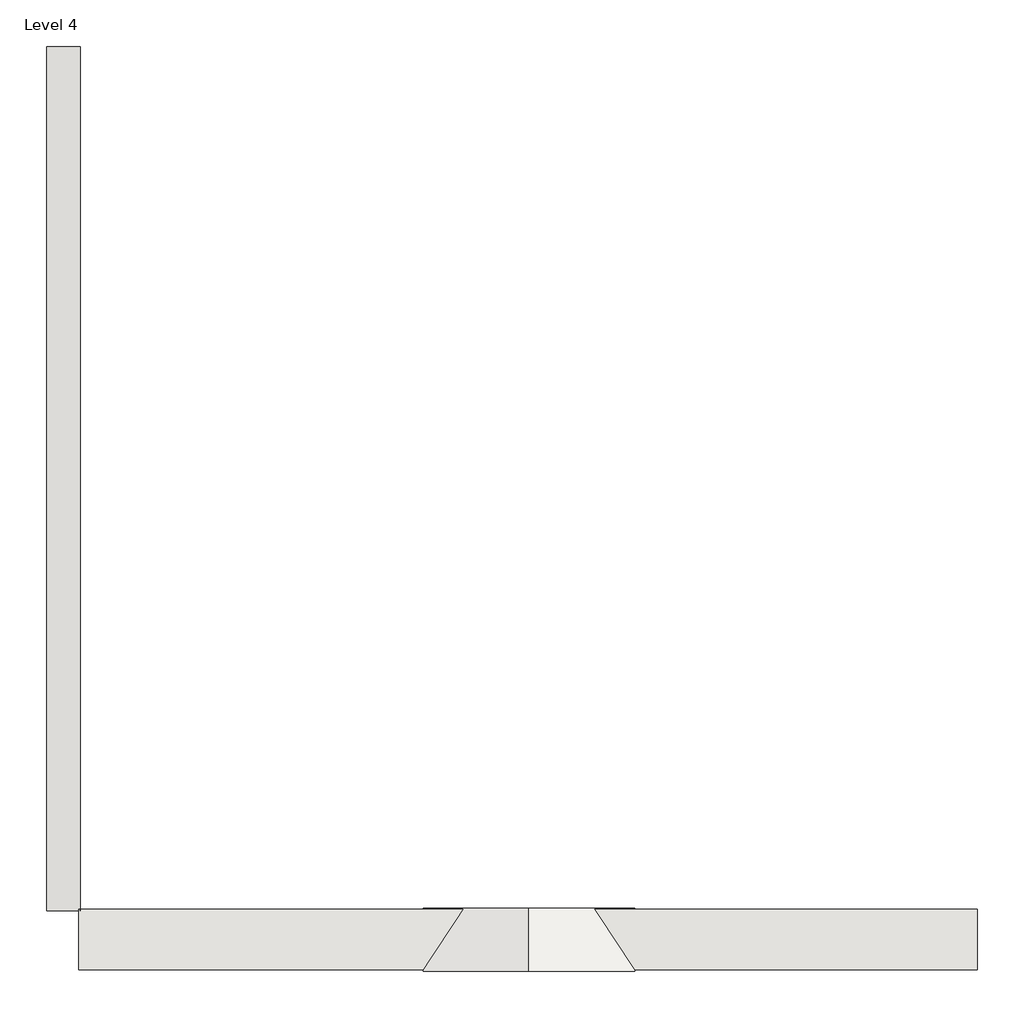
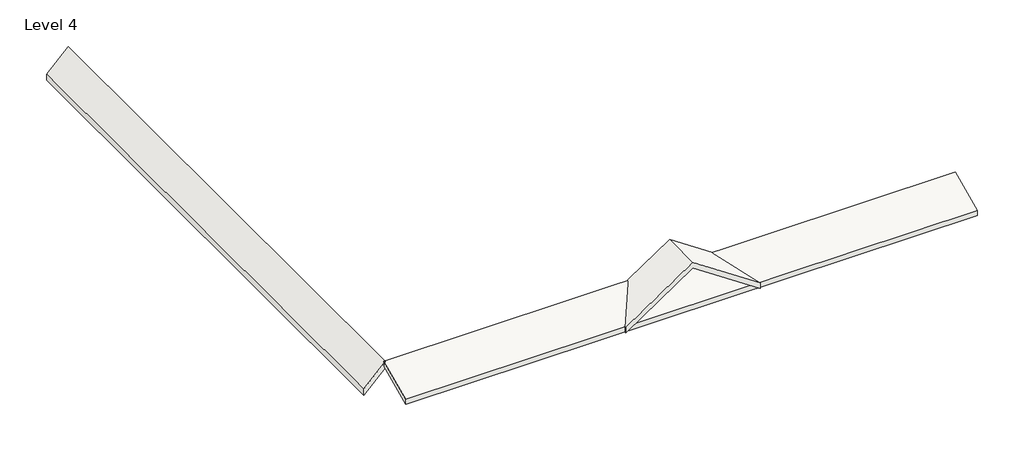
# One storey: 3 roofs.
"""IFC4 building model written with IfcOpenShell, lengths in millimetres."""

from ifc_helpers import new_model, si_unit, frame, origin, place, context, project, spatial, polyline, outline, extrude, element, save

model = new_model("IFC4")

# Units and contexts
model_context = context("Model", 3, world=origin())
ifc_project = project(units=[si_unit("LENGTHUNIT", "METRE", prefix="MILLI")], contexts=[model_context])

# Site, building, storey
site = spatial("IfcSite", under=ifc_project)
building = spatial("IfcBuilding", under=site)
storey = spatial("IfcBuildingStorey", under=building, Name="Level 4", Elevation=6858.0)

# Roofs
placement = place(None, origin())
element("IfcRoof", 1, ObjectType="6\" roof", at=placement, inside=storey, context=model_context, shape_type="SweptSolid", body=[
    extrude(outline(polyline([(-10080.7067839, 3252.1200204), (-8827.6878342, 3810.0), (-8827.6878342, 3643.1774312), (-10080.7067839, 3085.2974515), (-10080.7067839, 3252.1200204)])), frame((-9809.6634433, 0.0, 0.0), z_axis=(1.0, 0.0, 0.0), x_axis=(0.0, 1.0, 0.0)), (0.0, 0.0, 1.0), 18555.8213774),
])
element("IfcRoof", 2, ObjectType="6\" roof", at=placement, inside=storey, context=model_context, shape_type="SweptSolid", body=[
    extrude(outline(polyline([(3252.1200204, -2694.8868984), (3068.292405, -2694.8868984), (4540.5723846, -512.1420659), (3068.292405, 1670.6027667), (3252.1200204, 1670.6027667), (4724.4, -512.1420659), (3252.1200204, -2694.8868984)])), frame((0.0, -10112.12759, 0.0), z_axis=(0.0, 1.0, 0.0), x_axis=(0.0, 0.0, 1.0)), (0.0, 0.0, 1.0), 1298.9023851),
])
element("IfcRoof", 3, ObjectType="6\" roof", at=placement, inside=storey, context=model_context, shape_type="SweptSolid", body=[
    extrude(outline(polyline([(3109.5400226, -10470.9020433), (2894.0138757, -10470.9020433), (3594.4738531, -9770.4420659), (3810.0, -9770.4420659), (3109.5400226, -10470.9020433)])), frame((0.0, -8864.1469122, 0.0), z_axis=(0.0, 1.0, 0.0), x_axis=(0.0, 0.0, 1.0)), (0.0, 0.0, 1.0), 17841.859078),
])

save(model, "model.ifc")

# Revit data of these elements
# Type "6\" roof"
#   Assembly Code = "B1020"
#   Layers, outside or top first: 0' - 6" "roof balcony" (function 1)
# Elements 1, 2, 3 (IfcRoof, "6\" roof")
#   built-in parameter 1001710 = 33615
#   Phase Created = New Construction
#   Materials on its faces: "roof balcony"
# Materials
#   "roof balcony": class "Generic", colour RGB 120 120 120, transparency 0, Cost = 0
